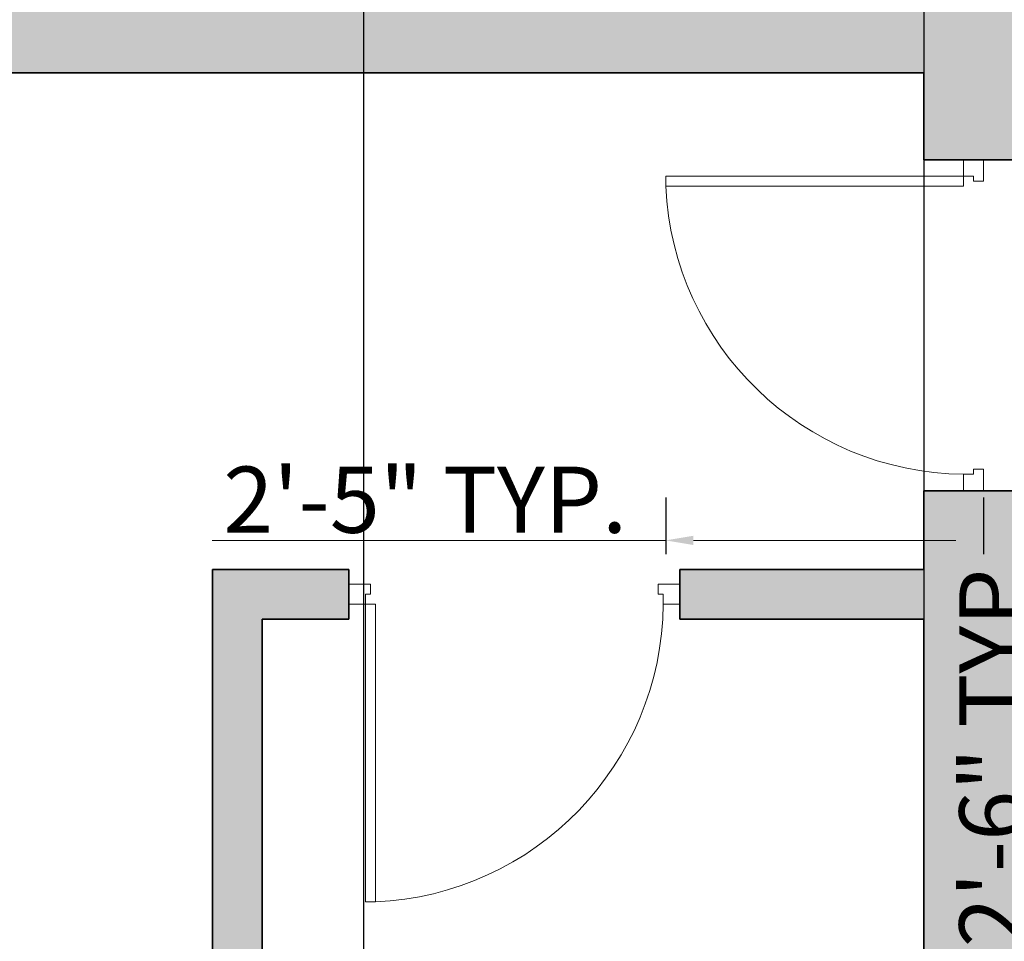
# Model space of a CAD drawing. Units: inches. Extents: x 2696 to 3240, y 1564 to 2310.
# Tile 12 of 76: x 2875 to 2964, y 1652 to 1736. Entities that reach past the tile are written whole.
import ezdxf

# ---------------------------------------------------------------- set-up
doc = ezdxf.new("R2010")
doc.units = ezdxf.units.IN
for name, color, linetype, lineweight in [('A-ANNO-DIMS', 3, 'Continuous', 18), ('A-DOOR', 4, 'Continuous', 18), ('A-WALL', 7, 'Continuous', 35), ('A-WALL-PATT', 9, 'Continuous', 13)]:
    doc.layers.add(name, color=color, linetype=linetype, lineweight=lineweight)
doc.styles.add('TIMES NEW', font='times.ttf')
doc.dimstyles.new('Siddhuu', dxfattribs={"dimtxt": 6, "dimasz": 2.5, "dimexe": 1.25, "dimexo": 0.625, "dimtad": 1, "dimdec": 1, "dimlunit": 4, "dimtxsty": 'TIMES NEW', "dimcen": 2.5, "dimclrd": 256, "dimclre": 1, "dimclrt": 7, "dimadec": 0, "dimazin": 0, "dimtfac": 1, "dimtdec": 1, "dimtmove": 0, "dimatfit": 3, "dimfxl": 1, "dimtolj": 1, "dimlwd": -1, "dimarcsym": 0})

# ---------------------------------------------------------------- blocks, each defined once
blk = doc.blocks.new('DR_D01')
for p, q in [((-0.45, 0.93), (-0.42, 0.93)), ((-0.45, 0.03), (-0.45, 0.93)), ((-0.42, 0.03), (-0.42, 0.93)), ((-0.5, 0.03), (-0.42, 0.03)), ((-0.5, 0.03), (-0.5, -0.03)), ((-0.45, 0.03), (-0.45, 0)), ((0.45, 0.03), (0.45, 0)), ((0.5, 0.03), (0.45, 0.03)), ((0.5, -0.03), (0.5, 0.03)), ((-0.45, 0), (-0.435, 0)), ((-0.435, 0), (-0.435, -0.03)), ((0.435, 0), (0.435, -0.03)), ((0.45, 0), (0.435, 0)), ((-0.435, -0.03), (-0.5, -0.03)), ((0.435, -0.03), (0.5, -0.03))]:
    blk.add_line(p, q)
blk.add_arc((-0.4602, 0.0206), 0.9103, 0.5915, 87.4664)
blk = doc.blocks.new('*D32')
at = {"layer": 'A-ANNO-DIMS', "color": 1, "lineweight": -2, "transparency": 16777216}
for p, q in [((2962.734, 1723.327), (2967.859, 1723.327)), ((2962.734, 1693.327), (2967.859, 1693.327))]:
    blk.add_line(p, q, dxfattribs=at)
at = {"layer": 'A-ANNO-DIMS', "transparency": 16777216}
for p, q in [((2966.609, 1720.827), (2966.609, 1695.827)), ((2966.609, 1693.327), (2966.609, 1624.849))]:
    blk.add_line(p, q, dxfattribs=at)
for points in [[(2966.192, 1720.827), (2967.025, 1720.827), (2966.609, 1723.327)], [(2966.192, 1695.827), (2967.025, 1695.827), (2966.609, 1693.327)]]:
    blk.add_solid(points, dxfattribs=at)
at = {"layer": 'Defpoints', "color": 0, "transparency": 16777216}
for p in [(2962.109, 1723.327), (2962.109, 1693.327), (2966.609, 1693.327)]:
    blk.add_point(p, dxfattribs=at)
at = {"layer": 'A-ANNO-DIMS', "color": 7, "transparency": 16777216, "insert": (2962.917, 1657.838), "char_height": 6, "attachment_point": 5, "rotation": 90, "style": 'TIMES NEW'}
blk.add_mtext('\\A1;DOOR 2\'-6" TYP.', dxfattribs=at)
blk = doc.blocks.new('*D33')
at = {"layer": 'A-ANNO-DIMS', "color": 1, "lineweight": -2, "transparency": 16777216}
for p, q in [((2933.309, 1692.702), (2933.309, 1687.577)), ((2962.109, 1692.702), (2962.109, 1687.577))]:
    blk.add_line(p, q, dxfattribs=at)
at = {"layer": 'A-ANNO-DIMS', "transparency": 16777216}
for p, q in [((2933.309, 1688.827), (2892.187, 1688.827)), ((2959.609, 1688.827), (2935.809, 1688.827))]:
    blk.add_line(p, q, dxfattribs=at)
for points in [[(2935.809, 1689.244), (2935.809, 1688.41), (2933.309, 1688.827)], [(2959.609, 1689.244), (2959.609, 1688.41), (2962.109, 1688.827)]]:
    blk.add_solid(points, dxfattribs=at)
at = {"layer": 'Defpoints', "color": 0, "transparency": 16777216}
for p in [(2933.309, 1693.327), (2962.109, 1693.327), (2933.309, 1688.827)]:
    blk.add_point(p, dxfattribs=at)
at = {"layer": 'A-ANNO-DIMS', "color": 7, "transparency": 16777216, "insert": (2911.498, 1692.513), "char_height": 6, "attachment_point": 5, "style": 'TIMES NEW'}
blk.add_mtext('\\A1;2\'-5" TYP.', dxfattribs=at)
blk = doc.blocks.new('*D57')
at = {"layer": 'A-ANNO-DIMS', "color": 1, "lineweight": -2, "transparency": 16777216}
for p, q in [((2754.611, 2018.576), (2754.611, 1568.951)), ((2956.709, 2018.576), (2956.709, 1568.951))]:
    blk.add_line(p, q, dxfattribs=at)
at = {"layer": 'A-ANNO-DIMS', "transparency": 16777216}
blk.add_line((2757.111, 1570.201), (2954.209, 1570.201), dxfattribs=at)
for points in [[(2757.111, 1570.618), (2757.111, 1569.784), (2754.611, 1570.201)], [(2954.209, 1570.618), (2954.209, 1569.784), (2956.709, 1570.201)]]:
    blk.add_solid(points, dxfattribs=at)
at = {"layer": 'Defpoints', "color": 0, "transparency": 16777216}
for p in [(2754.611, 2019.201), (2956.709, 2019.201), (2956.709, 1570.201)]:
    blk.add_point(p, dxfattribs=at)
at = {"layer": 'A-ANNO-DIMS', "color": 7, "transparency": 16777216, "insert": (2855.66, 1573.878), "char_height": 6, "attachment_point": 5, "style": 'TIMES NEW'}
blk.add_mtext('\\A1;16\'-10"', dxfattribs=at)
blk = doc.blocks.new('*D69')
at = {"layer": 'A-ANNO-DIMS', "color": 1, "lineweight": -2, "transparency": 16777216}
for p, q in [((2841.889, 2261.576), (2841.889, 1568.951)), ((2905.91, 2261.576), (2905.91, 1568.951))]:
    blk.add_line(p, q, dxfattribs=at)
at = {"layer": 'A-ANNO-DIMS', "transparency": 16777216}
blk.add_line((2844.389, 1570.201), (2903.41, 1570.201), dxfattribs=at)
for points in [[(2844.389, 1570.618), (2844.389, 1569.784), (2841.889, 1570.201)], [(2903.41, 1570.618), (2903.41, 1569.784), (2905.91, 1570.201)]]:
    blk.add_solid(points, dxfattribs=at)
at = {"layer": 'Defpoints', "color": 0, "transparency": 16777216}
for p in [(2841.889, 2262.201), (2905.91, 2262.201), (2905.91, 1570.201)]:
    blk.add_point(p, dxfattribs=at)
at = {"layer": 'A-ANNO-DIMS', "color": 7, "transparency": 16777216, "insert": (2873.9, 1573.878), "char_height": 6, "attachment_point": 5, "style": 'TIMES NEW'}
blk.add_mtext('\\A1;5\'-4"', dxfattribs=at)

msp = doc.modelspace()

# ---------------------------------------------------------------- hatches: boundary and pattern name
at = {"layer": 'A-WALL-PATT', "transparency": 33554556}
h = msp.add_hatch(color=256, dxfattribs=at)
h.dxf.hatch_style = 1
h.paths.add_polyline_path([(2879.111, 2253.201), (2905.91, 2253.201), (2905.91, 2262.201), (2841.889, 2262.201), (2841.889, 2253.201), (2870.111, 2253.201), (2870.111, 2176.601), (2965.709, 2176.601), (2965.709, 2206.701), (2973.583, 2206.701), (2973.583, 2215.701), (2965.709, 2215.701), (2965.709, 2262.201), (2929.91, 2262.201), (2929.91, 2253.201), (2956.709, 2253.201), (2956.709, 2185.601), (2879.111, 2185.601)])
h.paths.add_polyline_path([(2782.834, 2262.201), (2745.611, 2262.201), (2745.611, 2228.729), (2754.611, 2228.729), (2754.611, 2253.201), (2782.834, 2253.201)])
h.paths.add_polyline_path([(2754.611, 2136.201), (2965.709, 2136.201), (2965.709, 2145.201), (2879.111, 2145.201), (2879.111, 2147.074), (2877.34, 2147.074), (2870.111, 2147.074), (2870.111, 2145.201), (2754.611, 2145.201), (2754.611, 2169.674), (2745.611, 2169.674), (2745.611, 2000.201), (2754.611, 2000.201), (2754.611, 2019.201), (2849.083, 2019.201), (2849.083, 2023.701), (2841.209, 2023.701), (2841.209, 2051.827), (2836.709, 2051.827), (2836.709, 2023.701), (2754.611, 2023.701), (2754.611, 2091.201), (2836.709, 2091.201), (2836.709, 2087.827), (2841.209, 2087.827), (2841.209, 2095.701), (2754.611, 2095.701)])
h.paths.add_polyline_path([(2965.709, 2136.201), (2956.709, 2136.201), (2956.709, 2023.701), (2885.083, 2023.701), (2885.083, 2019.201), (2956.709, 2019.201), (2956.709, 1950.575), (2965.709, 1950.575), (2965.709, 1980.201), (2973.583, 1980.201), (2973.583, 1989.201), (2965.709, 1989.201)])
h.paths.add_polyline_path([(2754.611, 1906.701), (2880.209, 1906.701), (2884.709, 1906.701), (2956.709, 1906.701), (2956.709, 1792.701), (2944.709, 1792.701), (2944.709, 1783.701), (2956.709, 1783.701), (2956.709, 1740.201), (2884.709, 1740.201), (2884.709, 1783.701), (2896.709, 1783.701), (2896.709, 1792.701), (2884.709, 1792.701), (2884.709, 1846.701), (2880.209, 1846.701), (2880.209, 1740.201), (2754.611, 1740.201), (2754.611, 1777.201), (2745.611, 1777.201), (2745.611, 1692.701), (2754.611, 1692.701), (2754.611, 1731.201), (2956.709, 1731.201), (2956.709, 1723.327), (2965.709, 1723.327), (2965.709, 1884.201), (2973.583, 1884.201), (2973.583, 1893.201), (2965.709, 1893.201), (2965.709, 1914.575), (2956.709, 1914.575), (2956.709, 1911.201), (2754.611, 1911.201), (2754.611, 1930.201), (2745.611, 1930.201), (2745.611, 1817.201), (2754.611, 1817.201), (2754.611, 1854.201), (2826.611, 1854.201), (2826.611, 1868.827), (2822.111, 1868.827), (2822.111, 1858.701), (2754.611, 1858.701)])
h.paths.add_polyline_path([(2965.709, 1656.201), (3008.237, 1656.201), (3008.237, 1665.201), (2965.709, 1665.201), (2965.709, 1693.327), (2956.709, 1693.327), (2956.709, 1686.201), (2934.583, 1686.201), (2934.583, 1681.701), (2956.709, 1681.701), (2956.709, 1614.201), (2896.709, 1614.201), (2896.709, 1681.701), (2904.583, 1681.701), (2904.583, 1686.201), (2892.209, 1686.201), (2892.209, 1614.201), (2858.41, 1614.201), (2858.41, 1605.201), (2965.709, 1605.201)])
h.paths.add_polyline_path([(2788.41, 1614.201), (2754.611, 1614.201), (2754.611, 1652.701), (2745.611, 1652.701), (2745.611, 1605.201), (2788.41, 1605.201)])
h.paths.add_polyline_path([(3199.611, 1633.048), (3190.611, 1633.048), (3190.611, 1614.201), (3082.611, 1614.201), (3082.611, 1665.201), (3070.237, 1665.201), (3070.237, 1656.201), (3078.111, 1656.201), (3078.111, 1605.201), (3199.611, 1605.201)])
h.paths.add_polyline_path([(3199.611, 1702.048), (3190.611, 1702.048), (3190.611, 1699.701), (3106.611, 1699.701), (3106.611, 1747.701), (3190.611, 1747.701), (3190.611, 1752.201), (3082.611, 1752.201), (3082.611, 1760.075), (3078.111, 1760.075), (3078.111, 1747.701), (3102.111, 1747.701), (3102.111, 1699.701), (3078.111, 1699.701), (3078.111, 1695.201), (3190.611, 1695.201), (3190.611, 1676.355), (3199.611, 1676.355)])
h.paths.add_polyline_path([(3199.611, 1783.201), (3190.611, 1783.201), (3190.611, 1745.355), (3199.611, 1745.355)])
h.paths.add_polyline_path([(3082.611, 1884.201), (3190.611, 1884.201), (3190.611, 1853.201), (3199.611, 1853.201), (3199.611, 1901.701), (3190.611, 1901.701), (3190.611, 1893.201), (3005.583, 1893.201), (3005.583, 1891.281), (3005.583, 1884.201), (3078.111, 1884.201), (3078.111, 1792.075), (3082.611, 1792.075)])
h.paths.add_polyline_path([(3199.611, 1994.701), (3190.611, 1994.701), (3190.611, 1989.201), (3073.709, 1989.201), (3073.709, 2034.201), (3069.209, 2034.201), (3069.209, 1989.201), (3005.583, 1989.201), (3005.583, 1980.201), (3190.611, 1980.201), (3190.611, 1971.701), (3199.611, 1971.701)])
h.paths.add_polyline_path([(3199.611, 2155.201), (3190.611, 2155.201), (3190.611, 2064.701), (3199.611, 2064.701)])
h.paths.add_polyline_path([(3190.611, 2074.701), (3106.611, 2074.701), (3106.611, 2122.701), (3190.611, 2122.701), (3190.611, 2127.201), (3082.709, 2127.201), (3082.709, 2135.075), (3073.709, 2135.075), (3073.709, 2122.701), (3102.111, 2122.701), (3102.111, 2074.701), (3069.209, 2074.701), (3069.209, 2070.201), (3190.611, 2070.201)])
h.paths.add_polyline_path([(3082.709, 2253.201), (3190.611, 2253.201), (3190.611, 2225.201), (3199.611, 2225.201), (3199.611, 2262.201), (3073.709, 2262.201), (3073.709, 2215.701), (3035.583, 2215.701), (3035.583, 2206.701), (3073.709, 2206.701), (3073.709, 2171.075), (3082.709, 2171.075)])

# ---------------------------------------------------------------- linework, layer by layer
at = {"layer": 'A-WALL'}
for p, q in [((2754.611, 1731.201), (2956.709, 1731.201)), ((2956.709, 1731.201), (2956.709, 1723.327)), ((2956.709, 1723.327), (2965.709, 1723.327)), ((2956.709, 1693.327), (2956.709, 1686.201)), ((2956.709, 1693.327), (2965.709, 1693.327)), ((2892.209, 1686.201), (2904.583, 1686.201)), ((2892.209, 1686.201), (2892.209, 1614.201)), ((2904.583, 1681.701), (2904.583, 1686.201)), ((2934.583, 1686.201), (2956.709, 1686.201)), ((2934.583, 1681.701), (2934.583, 1686.201)), ((2896.709, 1681.701), (2896.709, 1614.201)), ((2896.709, 1681.701), (2904.583, 1681.701)), ((2934.583, 1681.701), (2956.709, 1681.701)), ((2956.709, 1681.701), (2956.709, 1614.201))]:
    msp.add_line(p, q, dxfattribs=at)

# ---------------------------------------------------------------- block references
at = {"layer": 'A-DOOR', "xscale": 30, "yscale": -30, "zscale": 30, "rotation": 269.9999999999948}
msp.add_blockref('DR_D01', (2961.209, 1708.327), dxfattribs=at)
at = {"layer": 'A-DOOR', "xscale": 30, "yscale": -30, "zscale": 30}
msp.add_blockref('DR_D01', (2919.583, 1683.951), dxfattribs=at)

# ---------------------------------------------------------------- dimensions: what is measured, and where the dimension line sits
at = {"layer": 'A-ANNO-DIMS'}
for base, p1, p2, picture, middle in [((2905.91, 1570.201), (2841.889, 2262.201), (2905.91, 2262.201), '*D69', (2873.9, 1573.878)), ((2956.709, 1570.201), (2754.611, 2019.201), (2956.709, 2019.201), '*D57', (2855.66, 1573.878))]:
    dim = msp.add_linear_dim(base=base, p1=p1, p2=p2, dimstyle='Siddhuu', override={"dimdec": 1, "dimlfac": 1, "dimrnd": 0, "dimzin": 1, "dimdsep": 46, "dimlunit": 4, "dimfrac": 2}, dxfattribs=at)
    dim.commit()
    dim.dimension.update_dxf_attribs({"geometry": picture, "text_midpoint": middle})
for base, p1, p2, angle, text, picture, middle in [((2966.609, 1693.327), (2962.109, 1723.327), (2962.109, 1693.327), 270, 'DOOR <> TYP.', '*D32', (2962.917, 1657.838)), ((2933.309, 1688.827), (2962.109, 1693.327), (2933.309, 1693.327), 180, '<> TYP.', '*D33', (2911.498, 1692.513))]:
    dim = msp.add_linear_dim(base=base, p1=p1, p2=p2, angle=angle, text=text, dimstyle='Siddhuu', override={"dimdec": 1, "dimlfac": 1, "dimrnd": 0, "dimzin": 1, "dimdsep": 46, "dimlunit": 4, "dimfrac": 2}, dxfattribs=at)
    dim.commit()
    dim.dimension.update_dxf_attribs({"geometry": picture, "text_midpoint": middle})

doc.saveas('drawing.dxf')
